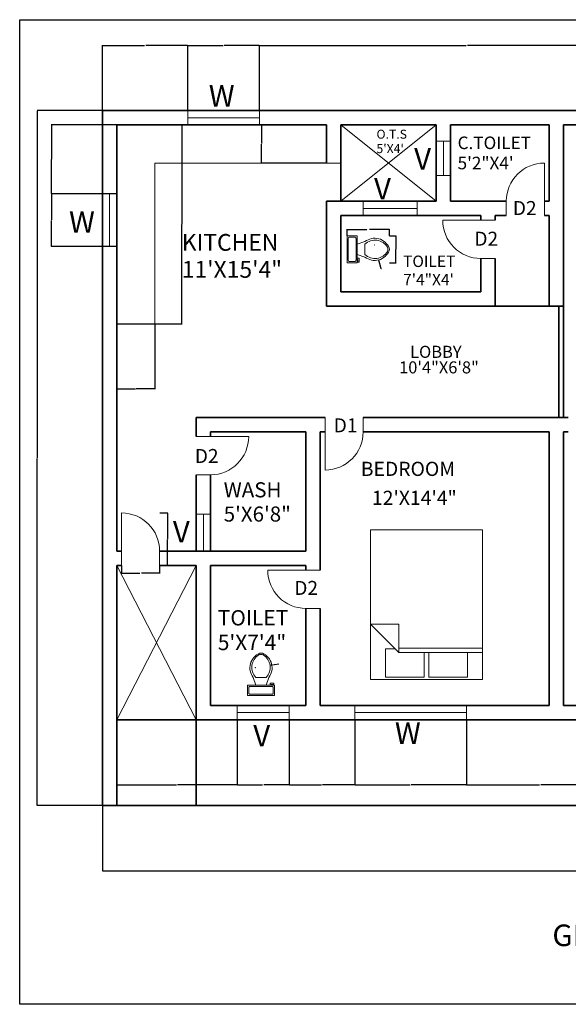
# Model space of a CAD drawing. Units: feet. Extents: x 1755 to 2628, y 1710 to 2329.
# Tile 1 of 4: x 1755 to 2100, y 1710 to 2329. Entities that reach past the tile are written whole.
import ezdxf

# ---------------------------------------------------------------- set-up
doc = ezdxf.new("R2010")
doc.units = ezdxf.units.FT
for name, color, linetype, lineweight in [('A-ANNO-DIMS', 2, 'Continuous', 18), ('A-ANNO-TEXT', 7, 'Continuous', 18), ('A-ANNO-TTLB', 7, 'Continuous', 25), ('A-AREA-IDEN', 7, 'Continuous', 18), ('A-DOOR', 3, 'Continuous', 18), ('A-FLOR-FIXT', 9, 'Continuous', 18), ('A-FLOR-OPEN', 8, 'Continuous', 13), ('A-FURN', 8, 'Continuous', 18), ('A-GLAZ', 4, 'Continuous', 18), ('A-WALL', 7, 'Continuous', 35)]:
    doc.layers.add(name, color=color, linetype=linetype, lineweight=lineweight)
doc.styles.get("Standard").update_dxf_attribs({"font": 'arial.ttf'})
doc.dimstyles.get("Standard").update_dxf_attribs({"dimtxt": 0.18, "dimasz": 0.18, "dimexe": 0.18, "dimexo": 0.0625, "dimgap": 0.09, "dimtad": 0, "dimtih": 1, "dimtoh": 1, "dimdec": 4, "dimzin": 0, "dimdsep": 46, "dimtxsty": 'Standard', "dimcen": 0.09, "dimadec": 0, "dimazin": 0, "dimtfac": 1, "dimtdec": 4, "dimtofl": 0, "dimtmove": 0, "dimatfit": 3, "dimfxl": 1, "dimtolj": 1, "dimtzin": 0, "dimarcsym": 0})

# ---------------------------------------------------------------- blocks, each defined once
blk = doc.blocks.new('Toilet - top')
for p, q in [((9.5, -6), (9.5, -2)), ((-10, -8.5), (-8, -8.5)), ((-10, -9.5), (-10, -8.5)), ((-7, -9.5), (-10, -9.5)), ((-8, -8.5), (-8, -8)), ((-7, -8), (-7, -9.5)), ((-4, -8), (-6, -14)), ((4, -14), (-4, -14)), ((4, -8), (6, -14))]:
    blk.add_line(p, q)
blk.add_lwpolyline([(10.5, -8), (10.5, 0), (-10.5, 0), (-10.5, -8)], close=True)
for points in [[(-9.5, -2), (-9.5, -6)], [(8.5, -1), (-8.5, -1)], [(-8.5, -7), (8.5, -7)]]:
    blk.add_lwpolyline(points)
for centre, radius, start, end in [((-8.62, -1.88), 0.884, 81.8699, 188.1301), ((-8.62, -6.12), 0.884, 171.8699, 278.1301), ((8.62, -1.88), 0.884, 351.8699, 98.1301), ((8.62, -6.12), 0.884, 261.8699, 8.1301), ((3.52, -21.58), 12.17, 141.46911, 247.97143), ((4.2, -21.82), 11.33, 136.36773, 238.94682), ((-3.52, -21.58), 12.17, 292.02843, 38.53071), ((-4.2, -21.82), 11.33, 301.05301, 43.63209), ((0, -27.88), 4, 245.73182, 294.26817), ((0, -29), 4, 254.86053, 285.13947)]:
    blk.add_arc(centre, radius, start, end)
blk = doc.blocks.new('Bed - Queen')
for p, q in [((0, -80.00003), (0, 0)), ((0, 0), (59.99999, 0)), ((59.99999, 0), (59.99999, -80.00003)), ((7.99999, -1.2), (28.79998, -1.2)), ((7.99999, -14.4), (7.99999, -1.2)), ((28.79998, -1.2), (28.79998, -14.4)), ((31.19999, -1.2), (51.99999, -1.2)), ((31.19999, -14.4), (31.19999, -1.2)), ((51.99999, -1.2), (51.99999, -16.4)), ((0, -14.4), (44.8, -14.4)), ((59.99999, -29.6), (44.8, -14.4)), ((44.8, -14.4), (44.8, -29.6)), ((44.8, -16.8), (0, -16.8)), ((51.99999, -16.4), (46.79936, -16.4)), ((44.8, -29.6), (59.99999, -29.6)), ((59.99999, -80.00003), (0, -80.00003))]:
    blk.add_line(p, q)
blk = doc.blocks.new('DOOR-SINGLE-SWING')
for p, q in [((0, 33), (0, 0)), ((24, 9), (24, 0))]:
    blk.add_line(p, q)
blk.add_arc((0, 9), 24, 0, 90)
blk = doc.blocks.new('*D8')
at = {"layer": 'A-ANNO-DIMS', "color": 0, "lineweight": -2, "transparency": 16777216}
for p, q in [((1842.95, 2018.82), (1848.02, 2018.82)), ((1847.84, 2018.64), (1847.84, 2002.5)), ((1847.84, 1986), (1847.84, 2002.13)), ((1842.95, 1985.82), (1848.02, 1985.82))]:
    blk.add_line(p, q, dxfattribs=at)
at = {"layer": 'A-ANNO-DIMS', "color": 0, "transparency": 16777216}
for points in [[(1847.81, 2018.64), (1847.87, 2018.64), (1847.84, 2018.82)], [(1847.81, 1986), (1847.87, 1986), (1847.84, 1985.82)]]:
    blk.add_solid(points, dxfattribs=at)
at = {"layer": 'Defpoints', "color": 0, "transparency": 16777216}
for p in [(1842.89, 2018.82), (1847.84, 2018.82), (1842.89, 1985.82)]:
    blk.add_point(p, dxfattribs=at)
at = {"layer": 'A-ANNO-DIMS', "color": 0, "transparency": 16777216, "insert": (1847.84, 2002.32), "char_height": 0.18, "attachment_point": 5}
blk.add_mtext('\\A1;SWING DOOR 33 TYP.', dxfattribs=at)
blk = doc.blocks.new('*D9')
at = {"layer": 'A-ANNO-DIMS', "color": 0, "lineweight": -2, "transparency": 16777216}
for p, q in [((1818.89, 1985.75), (1818.89, 1980.69)), ((1819.07, 1980.87), (1830.36, 1980.87)), ((1842.71, 1980.87), (1831.42, 1980.87)), ((1842.89, 1985.75), (1842.89, 1980.69))]:
    blk.add_line(p, q, dxfattribs=at)
at = {"layer": 'A-ANNO-DIMS', "color": 0, "transparency": 16777216}
for points in [[(1819.07, 1980.9), (1819.07, 1980.84), (1818.89, 1980.87)], [(1842.71, 1980.9), (1842.71, 1980.84), (1842.89, 1980.87)]]:
    blk.add_solid(points, dxfattribs=at)
at = {"layer": 'Defpoints', "color": 0, "transparency": 16777216}
for p in [(1818.89, 1985.82), (1842.89, 1985.82), (1842.89, 1980.87)]:
    blk.add_point(p, dxfattribs=at)
at = {"layer": 'A-ANNO-DIMS', "color": 0, "transparency": 16777216, "insert": (1830.89, 1980.87), "char_height": 0.18, "attachment_point": 5}
blk.add_mtext('\\A1;24 TYP.', dxfattribs=at)
blk = doc.blocks.new('*D12')
at = {"layer": 'A-ANNO-DIMS', "color": 0, "lineweight": -2, "transparency": 16777216}
for p, q in [((1960.72, 2193.1), (1960.72, 2197.22)), ((1960.9, 2197.04), (1973.28, 2197.04)), ((1987.22, 2197.04), (1974.84, 2197.04)), ((1987.4, 2193.1), (1987.4, 2197.22))]:
    blk.add_line(p, q, dxfattribs=at)
at = {"layer": 'A-ANNO-DIMS', "color": 0, "transparency": 16777216}
for points in [[(1960.9, 2197.07), (1960.9, 2197.01), (1960.72, 2197.04)], [(1987.22, 2197.07), (1987.22, 2197.01), (1987.4, 2197.04)]]:
    blk.add_solid(points, dxfattribs=at)
at = {"layer": 'Defpoints', "color": 0, "transparency": 16777216}
for p in [(1960.72, 2197.04), (1960.72, 2193.04), (1987.4, 2193.04)]:
    blk.add_point(p, dxfattribs=at)
at = {"layer": 'A-ANNO-DIMS', "color": 0, "transparency": 16777216, "insert": (1974.06, 2197.04), "char_height": 0.18, "attachment_point": 5}
blk.add_mtext('\\A1;WC 27 TYP.', dxfattribs=at)
blk = doc.blocks.new('*D13')
at = {"layer": 'A-ANNO-DIMS', "color": 0, "lineweight": -2, "transparency": 16777216}
for p, q in [((1987.47, 2193.04), (1991.58, 2193.04)), ((1991.4, 2192.86), (1991.4, 2184.74)), ((1991.4, 2176.26), (1991.4, 2184.38)), ((1987.47, 2176.08), (1991.58, 2176.08))]:
    blk.add_line(p, q, dxfattribs=at)
at = {"layer": 'A-ANNO-DIMS', "color": 0, "transparency": 16777216}
for points in [[(1991.37, 2192.86), (1991.43, 2192.86), (1991.4, 2193.04)], [(1991.37, 2176.26), (1991.43, 2176.26), (1991.4, 2176.08)]]:
    blk.add_solid(points, dxfattribs=at)
at = {"layer": 'Defpoints', "color": 0, "transparency": 16777216}
for p in [(1987.4, 2193.04), (1991.4, 2193.04), (1987.4, 2176.08)]:
    blk.add_point(p, dxfattribs=at)
at = {"layer": 'A-ANNO-DIMS', "color": 0, "transparency": 16777216, "insert": (1991.4, 2184.56), "char_height": 0.18, "attachment_point": 5}
blk.add_mtext('\\A1;17 TYP.', dxfattribs=at)
blk = doc.blocks.new('*D22')
at = {"layer": 'A-ANNO-DIMS', "color": 0, "lineweight": -2, "transparency": 16777216}
for p, q in [((1806.89, 1834.75), (1806.89, 1793.69)), ((2548.89, 1834.75), (2548.89, 1793.69)), ((1807.07, 1793.87), (2177.6, 1793.87)), ((2548.71, 1793.87), (2178.18, 1793.87))]:
    blk.add_line(p, q, dxfattribs=at)
at = {"layer": 'A-ANNO-DIMS', "color": 0, "transparency": 16777216}
for points in [[(1807.07, 1793.9), (1807.07, 1793.84), (1806.89, 1793.87)], [(2548.71, 1793.9), (2548.71, 1793.84), (2548.89, 1793.87)]]:
    blk.add_solid(points, dxfattribs=at)
at = {"layer": 'Defpoints', "color": 0, "transparency": 16777216}
for p in [(1806.89, 1834.82), (2548.89, 1834.82), (2548.89, 1793.87)]:
    blk.add_point(p, dxfattribs=at)
at = {"layer": 'A-ANNO-DIMS', "color": 0, "transparency": 16777216, "insert": (2177.89, 1793.87), "char_height": 0.18, "attachment_point": 5}
blk.add_mtext('\\A1;742', dxfattribs=at)
blk = doc.blocks.new('*D23')
at = {"layer": 'A-ANNO-DIMS', "color": 0, "lineweight": -2, "transparency": 16777216}
for p, q in [((1806.83, 2271.82), (1765.76, 2271.82)), ((1765.94, 2271.64), (1765.94, 2053.5)), ((1765.94, 1835), (1765.94, 2053.13)), ((1806.83, 1834.82), (1765.76, 1834.82))]:
    blk.add_line(p, q, dxfattribs=at)
at = {"layer": 'A-ANNO-DIMS', "color": 0, "transparency": 16777216}
for points in [[(1765.91, 2271.64), (1765.97, 2271.64), (1765.94, 2271.82)], [(1765.91, 1835), (1765.97, 1835), (1765.94, 1834.82)]]:
    blk.add_solid(points, dxfattribs=at)
at = {"layer": 'Defpoints', "color": 0, "transparency": 16777216}
for p in [(1765.94, 2271.82), (1806.89, 2271.82), (1806.89, 1834.82)]:
    blk.add_point(p, dxfattribs=at)
at = {"layer": 'A-ANNO-DIMS', "color": 0, "transparency": 16777216, "insert": (1765.94, 2053.32), "char_height": 0.18, "attachment_point": 5}
blk.add_mtext('\\A1;437', dxfattribs=at)
blk = doc.blocks.new('*D24')
at = {"layer": 'A-ANNO-DIMS', "color": 0, "lineweight": -2, "transparency": 16777216}
for p, q in [((1806.89, 2271.88), (1806.89, 2312.95)), ((1807.07, 2312.77), (1833.36, 2312.77)), ((1860.43, 2312.77), (1834.14, 2312.77)), ((1860.61, 2271.88), (1860.61, 2312.95))]:
    blk.add_line(p, q, dxfattribs=at)
at = {"layer": 'A-ANNO-DIMS', "color": 0, "transparency": 16777216}
for points in [[(1807.07, 2312.8), (1807.07, 2312.74), (1806.89, 2312.77)], [(1860.43, 2312.8), (1860.43, 2312.74), (1860.61, 2312.77)]]:
    blk.add_solid(points, dxfattribs=at)
at = {"layer": 'Defpoints', "color": 0, "transparency": 16777216}
for p in [(1860.61, 2312.77), (1806.89, 2271.82), (1860.61, 2271.82)]:
    blk.add_point(p, dxfattribs=at)
at = {"layer": 'A-ANNO-DIMS', "color": 0, "transparency": 16777216, "insert": (1833.75, 2312.77), "char_height": 0.18, "attachment_point": 5}
blk.add_mtext('\\A1;53.72', dxfattribs=at)
blk = doc.blocks.new('*D25')
at = {"layer": 'A-ANNO-DIMS', "color": 0, "lineweight": -2, "transparency": 16777216}
for p, q in [((1860.61, 2271.88), (1860.61, 2312.95)), ((1860.79, 2312.77), (1882.75, 2312.77)), ((1905.51, 2312.77), (1883.55, 2312.77)), ((1905.69, 2271.88), (1905.69, 2312.95))]:
    blk.add_line(p, q, dxfattribs=at)
at = {"layer": 'A-ANNO-DIMS', "color": 0, "transparency": 16777216}
for points in [[(1860.79, 2312.8), (1860.79, 2312.74), (1860.61, 2312.77)], [(1905.51, 2312.8), (1905.51, 2312.74), (1905.69, 2312.77)]]:
    blk.add_solid(points, dxfattribs=at)
at = {"layer": 'Defpoints', "color": 0, "transparency": 16777216}
for p in [(1905.69, 2312.77), (1860.61, 2271.82), (1905.69, 2271.82)]:
    blk.add_point(p, dxfattribs=at)
at = {"layer": 'A-ANNO-DIMS', "color": 0, "transparency": 16777216, "insert": (1883.15, 2312.77), "char_height": 0.18, "attachment_point": 5}
blk.add_mtext('\\A1;45.07', dxfattribs=at)
blk = doc.blocks.new('*D26')
at = {"layer": 'A-ANNO-DIMS', "color": 0, "lineweight": -2, "transparency": 16777216}
for p, q in [((1905.69, 2271.88), (1905.69, 2312.95)), ((1905.87, 2312.77), (2035.59, 2312.77)), ((2166.25, 2312.77), (2036.53, 2312.77)), ((2166.43, 2271.88), (2166.43, 2312.95))]:
    blk.add_line(p, q, dxfattribs=at)
at = {"layer": 'A-ANNO-DIMS', "color": 0, "transparency": 16777216}
for points in [[(1905.87, 2312.8), (1905.87, 2312.74), (1905.69, 2312.77)], [(2166.25, 2312.8), (2166.25, 2312.74), (2166.43, 2312.77)]]:
    blk.add_solid(points, dxfattribs=at)
at = {"layer": 'Defpoints', "color": 0, "transparency": 16777216}
for p in [(2166.43, 2312.77), (1905.69, 2271.82), (2166.43, 2271.82)]:
    blk.add_point(p, dxfattribs=at)
at = {"layer": 'A-ANNO-DIMS', "color": 0, "transparency": 16777216, "insert": (2036.06, 2312.77), "char_height": 0.18, "attachment_point": 5}
blk.add_mtext('\\A1;260.75', dxfattribs=at)
blk = doc.blocks.new('*D36')
at = {"layer": 'A-ANNO-DIMS', "color": 0, "lineweight": -2, "transparency": 16777216}
for p, q in [((1815.89, 1888.75), (1815.89, 1847.69)), ((1891.73, 1888.75), (1891.73, 1847.69)), ((1816.07, 1847.87), (1853.42, 1847.87)), ((1891.55, 1847.87), (1854.2, 1847.87))]:
    blk.add_line(p, q, dxfattribs=at)
at = {"layer": 'A-ANNO-DIMS', "color": 0, "transparency": 16777216}
for points in [[(1816.07, 1847.9), (1816.07, 1847.84), (1815.89, 1847.87)], [(1891.55, 1847.9), (1891.55, 1847.84), (1891.73, 1847.87)]]:
    blk.add_solid(points, dxfattribs=at)
at = {"layer": 'Defpoints', "color": 0, "transparency": 16777216}
for p in [(1815.89, 1888.82), (1891.73, 1888.82), (1815.89, 1847.87)]:
    blk.add_point(p, dxfattribs=at)
at = {"layer": 'A-ANNO-DIMS', "color": 0, "transparency": 16777216, "insert": (1853.81, 1847.87), "char_height": 0.18, "attachment_point": 5}
blk.add_mtext('\\A1;75.84', dxfattribs=at)
blk = doc.blocks.new('*D37')
at = {"layer": 'A-ANNO-DIMS', "color": 0, "lineweight": -2, "transparency": 16777216}
for p, q in [((1891.73, 1888.75), (1891.73, 1847.69)), ((1924.29, 1888.75), (1924.29, 1847.69)), ((1891.91, 1847.87), (1907.62, 1847.87)), ((1924.11, 1847.87), (1908.4, 1847.87))]:
    blk.add_line(p, q, dxfattribs=at)
at = {"layer": 'A-ANNO-DIMS', "color": 0, "transparency": 16777216}
for points in [[(1891.91, 1847.9), (1891.91, 1847.84), (1891.73, 1847.87)], [(1924.11, 1847.9), (1924.11, 1847.84), (1924.29, 1847.87)]]:
    blk.add_solid(points, dxfattribs=at)
at = {"layer": 'Defpoints', "color": 0, "transparency": 16777216}
for p in [(1891.73, 1888.82), (1924.29, 1888.82), (1891.73, 1847.87)]:
    blk.add_point(p, dxfattribs=at)
at = {"layer": 'A-ANNO-DIMS', "color": 0, "transparency": 16777216, "insert": (1908.01, 1847.87), "char_height": 0.18, "attachment_point": 5}
blk.add_mtext('\\A1;32.56', dxfattribs=at)
blk = doc.blocks.new('*D38')
at = {"layer": 'A-ANNO-DIMS', "color": 0, "lineweight": -2, "transparency": 16777216}
for p, q in [((1924.29, 1888.75), (1924.29, 1847.69)), ((1965.72, 1888.75), (1965.72, 1847.69)), ((1924.47, 1847.87), (1944.61, 1847.87)), ((1965.54, 1847.87), (1945.4, 1847.87))]:
    blk.add_line(p, q, dxfattribs=at)
at = {"layer": 'A-ANNO-DIMS', "color": 0, "transparency": 16777216}
for points in [[(1924.47, 1847.9), (1924.47, 1847.84), (1924.29, 1847.87)], [(1965.54, 1847.9), (1965.54, 1847.84), (1965.72, 1847.87)]]:
    blk.add_solid(points, dxfattribs=at)
at = {"layer": 'Defpoints', "color": 0, "transparency": 16777216}
for p in [(1924.29, 1888.82), (1965.72, 1888.82), (1924.29, 1847.87)]:
    blk.add_point(p, dxfattribs=at)
at = {"layer": 'A-ANNO-DIMS', "color": 0, "transparency": 16777216, "insert": (1945, 1847.87), "char_height": 0.18, "attachment_point": 5}
blk.add_mtext('\\A1;41.43', dxfattribs=at)
blk = doc.blocks.new('*D39')
at = {"layer": 'A-ANNO-DIMS', "color": 0, "lineweight": -2, "transparency": 16777216}
for p, q in [((1965.72, 1888.75), (1965.72, 1847.69)), ((2035.77, 1888.75), (2035.77, 1847.69)), ((1965.9, 1847.87), (2000.35, 1847.87)), ((2035.59, 1847.87), (2001.14, 1847.87))]:
    blk.add_line(p, q, dxfattribs=at)
at = {"layer": 'A-ANNO-DIMS', "color": 0, "transparency": 16777216}
for points in [[(1965.9, 1847.9), (1965.9, 1847.84), (1965.72, 1847.87)], [(2035.59, 1847.9), (2035.59, 1847.84), (2035.77, 1847.87)]]:
    blk.add_solid(points, dxfattribs=at)
at = {"layer": 'Defpoints', "color": 0, "transparency": 16777216}
for p in [(1965.72, 1888.82), (2035.77, 1888.82), (1965.72, 1847.87)]:
    blk.add_point(p, dxfattribs=at)
at = {"layer": 'A-ANNO-DIMS', "color": 0, "transparency": 16777216, "insert": (2000.75, 1847.87), "char_height": 0.18, "attachment_point": 5}
blk.add_mtext('\\A1;70.06', dxfattribs=at)
blk = doc.blocks.new('*D40')
at = {"layer": 'A-ANNO-DIMS', "color": 0, "lineweight": -2, "transparency": 16777216}
for p, q in [((2035.77, 1888.75), (2035.77, 1847.69)), ((2128.5, 1888.75), (2128.5, 1847.69)), ((2035.95, 1847.87), (2081.75, 1847.87)), ((2128.32, 1847.87), (2082.53, 1847.87))]:
    blk.add_line(p, q, dxfattribs=at)
at = {"layer": 'A-ANNO-DIMS', "color": 0, "transparency": 16777216}
for points in [[(2035.95, 1847.9), (2035.95, 1847.84), (2035.77, 1847.87)], [(2128.32, 1847.9), (2128.32, 1847.84), (2128.5, 1847.87)]]:
    blk.add_solid(points, dxfattribs=at)
at = {"layer": 'Defpoints', "color": 0, "transparency": 16777216}
for p in [(2035.77, 1888.82), (2128.5, 1888.82), (2035.77, 1847.87)]:
    blk.add_point(p, dxfattribs=at)
at = {"layer": 'A-ANNO-DIMS', "color": 0, "transparency": 16777216, "insert": (2082.14, 1847.87), "char_height": 0.18, "attachment_point": 5}
blk.add_mtext('\\A1;92.73', dxfattribs=at)
blk = doc.blocks.new('*D49')
at = {"layer": 'A-ANNO-DIMS', "color": 0, "lineweight": -2, "transparency": 16777216}
for p, q in [((1815.83, 2219.52), (1774.76, 2219.52)), ((1774.94, 2219.34), (1774.94, 2203.14)), ((1774.94, 2186.58), (1774.94, 2202.78)), ((1815.83, 2186.4), (1774.76, 2186.4))]:
    blk.add_line(p, q, dxfattribs=at)
at = {"layer": 'A-ANNO-DIMS', "color": 0, "transparency": 16777216}
for points in [[(1774.91, 2219.34), (1774.97, 2219.34), (1774.94, 2219.52)], [(1774.91, 2186.58), (1774.97, 2186.58), (1774.94, 2186.4)]]:
    blk.add_solid(points, dxfattribs=at)
at = {"layer": 'Defpoints', "color": 0, "transparency": 16777216}
for p in [(1774.94, 2219.52), (1815.89, 2219.52), (1815.89, 2186.4)]:
    blk.add_point(p, dxfattribs=at)
at = {"layer": 'A-ANNO-DIMS', "color": 0, "transparency": 16777216, "insert": (1774.94, 2202.96), "char_height": 0.18, "attachment_point": 5}
blk.add_mtext('\\A1;33.12', dxfattribs=at)
blk = doc.blocks.new('*D50')
at = {"layer": 'A-ANNO-DIMS', "color": 0, "lineweight": -2, "transparency": 16777216}
for p, q in [((1815.83, 2262.82), (1774.76, 2262.82)), ((1774.94, 2262.64), (1774.94, 2241.35)), ((1774.94, 2219.7), (1774.94, 2240.98)), ((1815.83, 2219.52), (1774.76, 2219.52))]:
    blk.add_line(p, q, dxfattribs=at)
at = {"layer": 'A-ANNO-DIMS', "color": 0, "transparency": 16777216}
for points in [[(1774.91, 2262.64), (1774.97, 2262.64), (1774.94, 2262.82)], [(1774.91, 2219.7), (1774.97, 2219.7), (1774.94, 2219.52)]]:
    blk.add_solid(points, dxfattribs=at)
at = {"layer": 'Defpoints', "color": 0, "transparency": 16777216}
for p in [(1774.94, 2262.82), (1815.89, 2262.82), (1815.89, 2219.52)]:
    blk.add_point(p, dxfattribs=at)
at = {"layer": 'A-ANNO-DIMS', "color": 0, "transparency": 16777216, "insert": (1774.94, 2241.17), "char_height": 0.18, "attachment_point": 5}
blk.add_mtext('\\A1;43.3', dxfattribs=at)
blk = doc.blocks.new('*D51')
at = {"layer": 'A-ANNO-DIMS', "color": 0, "lineweight": -2, "transparency": 16777216}
for p, q in [((1815.89, 2137.71), (1815.89, 2096.64)), ((1839.89, 2137.71), (1839.89, 2096.64)), ((1816.07, 2096.82), (1827.67, 2096.82)), ((1839.71, 2096.82), (1828.11, 2096.82))]:
    blk.add_line(p, q, dxfattribs=at)
at = {"layer": 'A-ANNO-DIMS', "color": 0, "transparency": 16777216}
for points in [[(1816.07, 2096.85), (1816.07, 2096.79), (1815.89, 2096.82)], [(1839.71, 2096.85), (1839.71, 2096.79), (1839.89, 2096.82)]]:
    blk.add_solid(points, dxfattribs=at)
at = {"layer": 'Defpoints', "color": 0, "transparency": 16777216}
for p in [(1815.89, 2137.77), (1839.89, 2137.77), (1815.89, 2096.82)]:
    blk.add_point(p, dxfattribs=at)
at = {"layer": 'A-ANNO-DIMS', "color": 0, "transparency": 16777216, "insert": (1827.89, 2096.82), "char_height": 0.18, "attachment_point": 5}
blk.add_mtext('\\A1;24', dxfattribs=at)
blk = doc.blocks.new('*D52')
at = {"layer": 'A-ANNO-DIMS', "color": 0, "lineweight": -2, "transparency": 16777216}
for p, q in [((1815.95, 2262.82), (1857.02, 2262.82)), ((1856.84, 2262.64), (1856.84, 2200.48)), ((1856.84, 2137.95), (1856.84, 2200.11)), ((1815.95, 2137.77), (1857.02, 2137.77))]:
    blk.add_line(p, q, dxfattribs=at)
at = {"layer": 'A-ANNO-DIMS', "color": 0, "transparency": 16777216}
for points in [[(1856.81, 2262.64), (1856.87, 2262.64), (1856.84, 2262.82)], [(1856.81, 2137.95), (1856.87, 2137.95), (1856.84, 2137.77)]]:
    blk.add_solid(points, dxfattribs=at)
at = {"layer": 'Defpoints', "color": 0, "transparency": 16777216}
for p in [(1815.89, 2262.82), (1815.89, 2137.77), (1856.84, 2137.77)]:
    blk.add_point(p, dxfattribs=at)
at = {"layer": 'A-ANNO-DIMS', "color": 0, "transparency": 16777216, "insert": (1856.84, 2200.3), "char_height": 0.18, "attachment_point": 5}
blk.add_mtext('\\A1;125.04', dxfattribs=at)
blk = doc.blocks.new('*D53')
at = {"layer": 'A-ANNO-DIMS', "color": 0, "lineweight": -2, "transparency": 16777216}
for p, q in [((1947.83, 2262.82), (1906.76, 2262.82)), ((1906.94, 2262.64), (1906.94, 2251)), ((1906.94, 2239), (1906.94, 2250.64)), ((1947.83, 2238.82), (1906.76, 2238.82))]:
    blk.add_line(p, q, dxfattribs=at)
at = {"layer": 'A-ANNO-DIMS', "color": 0, "transparency": 16777216}
for points in [[(1906.91, 2262.64), (1906.97, 2262.64), (1906.94, 2262.82)], [(1906.91, 2239), (1906.97, 2239), (1906.94, 2238.82)]]:
    blk.add_solid(points, dxfattribs=at)
at = {"layer": 'Defpoints', "color": 0, "transparency": 16777216}
for p in [(1906.94, 2262.82), (1947.89, 2262.82), (1947.89, 2238.82)]:
    blk.add_point(p, dxfattribs=at)
at = {"layer": 'A-ANNO-DIMS', "color": 0, "transparency": 16777216, "insert": (1906.94, 2250.82), "char_height": 0.18, "attachment_point": 5}
blk.add_mtext('\\A1;24', dxfattribs=at)
blk = doc.blocks.new('*D59')
at = {"layer": 'A-ANNO-DIMS', "color": 0, "lineweight": -2, "transparency": 16777216}
for p, q in [((1978.05, 2187.4), (1978.23, 2187.4)), ((1978.14, 2187.31), (1978.14, 2187.49)), ((1982.14, 2172.2), (1980.69, 2177.73)), ((1982.32, 2172.2), (1982.14, 2172.2))]:
    blk.add_line(p, q, dxfattribs=at)
at = {"layer": 'A-ANNO-DIMS', "color": 0, "transparency": 16777216}
blk.add_solid([(1980.72, 2177.73), (1980.66, 2177.72), (1980.64, 2177.9)], dxfattribs=at)
at = {"layer": 'Defpoints', "color": 0, "transparency": 16777216}
for p in [(1978.14, 2187.4), (1980.64, 2177.9)]:
    blk.add_point(p, dxfattribs=at)
at = {"layer": 'A-ANNO-DIMS', "color": 0, "transparency": 16777216, "insert": (1983, 2172.2), "char_height": 0.18, "attachment_point": 5}
blk.add_mtext('\\A1;4X R9.826', dxfattribs=at)
blk = doc.blocks.new('*D60')
at = {"layer": 'A-ANNO-DIMS', "color": 0, "lineweight": -2, "transparency": 16777216}
for p, q in [((1903.16, 1921.71), (1903.34, 1921.71)), ((1903.25, 1921.62), (1903.25, 1921.8)), ((1917.75, 1923.66), (1912.49, 1922.96))]:
    blk.add_line(p, q, dxfattribs=at)
at = {"layer": 'A-ANNO-DIMS', "color": 0, "transparency": 16777216}
blk.add_solid([(1912.49, 1922.99), (1912.5, 1922.93), (1912.31, 1922.93)], dxfattribs=at)
at = {"layer": 'Defpoints', "color": 0, "transparency": 16777216}
for p in [(1903.25, 1921.71), (1912.31, 1922.93)]:
    blk.add_point(p, dxfattribs=at)
at = {"layer": 'A-ANNO-DIMS', "color": 0, "transparency": 16777216, "insert": (1918.43, 1923.66), "char_height": 0.18, "attachment_point": 5}
blk.add_mtext('\\A1;4X R9.148', dxfattribs=at)

msp = doc.modelspace()

# ---------------------------------------------------------------- linework, layer by layer
at = {"layer": 'A-ANNO-TTLB'}
msp.add_lwpolyline([(1754.8706, 2328.9307), (2627.7013, 2328.9307), (2627.7013, 1709.9251), (1754.8706, 1709.9251)], close=True, dxfattribs=at)
at = {"layer": 'A-FLOR-FIXT'}
for p, q in [((1839.8905, 2238.8157), (1956.8905, 2238.8157)), ((1839.8905, 2137.7746), (1839.8905, 2238.8157)), ((1815.8905, 2137.7746), (1839.8905, 2137.7746))]:
    msp.add_line(p, q, dxfattribs=at)
at = {"layer": 'A-FLOR-OPEN'}
for p, q in [((1956.8905, 2262.8157), (2016.8905, 2214.8157)), ((1956.8905, 2214.8157), (2016.8905, 2262.8157)), ((1815.8905, 1985.8157), (1865.8905, 1888.8157)), ((1865.8905, 1985.8157), (1815.8905, 1888.8157))]:
    msp.add_line(p, q, dxfattribs=at)
at = {"layer": 'A-GLAZ'}
for p, q in [((1860.6124, 2271.8157), (1860.6124, 2262.8157)), ((1905.6851, 2271.8157), (1905.6851, 2262.8157)), ((1860.6124, 2267.3157), (1905.6851, 2267.3157)), ((2016.8905, 2252.4841), (2025.8905, 2252.4841)), ((2021.3905, 2252.4841), (2021.3905, 2230.9614)), ((2016.8905, 2230.9614), (2025.8905, 2230.9614)), ((1806.8905, 2219.5181), (1815.8905, 2219.5181)), ((1811.3905, 2219.5181), (1811.3905, 2186.3991)), ((1970.8608, 2214.8157), (1970.8608, 2205.8157)), ((1970.8608, 2210.3157), (2004.908, 2210.3157)), ((2004.908, 2214.8157), (2004.908, 2205.8157)), ((1806.8905, 2186.3991), (1815.8905, 2186.3991)), ((1865.8905, 2018.1107), (1874.8905, 2018.1107)), ((1870.3905, 2018.1107), (1870.3905, 1994.8157)), ((1891.7318, 1897.8157), (1891.7318, 1888.8157)), ((1924.2905, 1897.8157), (1924.2905, 1888.8157)), ((1965.7178, 1897.8157), (1965.7178, 1888.8157)), ((2035.7745, 1897.8157), (2035.7745, 1888.8157)), ((1891.7318, 1893.3157), (1924.2905, 1893.3157)), ((1965.7178, 1893.3157), (2035.7745, 1893.3157))]:
    msp.add_line(p, q, dxfattribs=at)
at = {"layer": 'A-WALL'}
for p, q in [((1806.8905, 2271.8157), (1947.8905, 2271.8157)), ((1806.8905, 2078.8157), (1806.8905, 2271.8157)), ((1806.8905, 2271.8157), (2096.8905, 2271.8157)), ((2025.8905, 2271.8157), (2096.8905, 2271.8157)), ((2096.8905, 2271.8157), (2548.8905, 2271.8157)), ((1815.8905, 2262.8157), (1947.8905, 2262.8157)), ((1815.8905, 2069.8157), (1815.8905, 2262.8157)), ((1947.8905, 2262.8157), (1947.8905, 2238.8157)), ((1956.8905, 2262.8157), (1956.8905, 2214.8157)), ((1956.8905, 2262.8157), (2016.8905, 2262.8157)), ((2016.8905, 2262.8157), (2016.8905, 2214.8157)), ((2025.8905, 2262.8157), (2025.8905, 2214.8157)), ((2025.8905, 2262.8157), (2087.8905, 2262.8157)), ((2087.8905, 2262.8157), (2087.8905, 2214.8157)), ((2096.8905, 2262.8157), (2096.8905, 2214.8157)), ((2096.8905, 2262.8157), (2378.8905, 2262.8157)), ((2016.8905, 2214.8157), (1947.8905, 2214.8157)), ((1947.8905, 2214.8157), (1947.8905, 2148.8157)), ((1956.8905, 2214.8157), (2016.8905, 2214.8157)), ((2060.8905, 2214.8157), (2025.8905, 2214.8157)), ((2087.8905, 2214.8157), (2084.8905, 2214.8157)), ((2096.8905, 2214.8157), (2096.8905, 2078.8157)), ((1956.8905, 2205.8157), (1956.8905, 2157.8157)), ((1956.8905, 2205.8157), (2044.8905, 2205.8157)), ((2044.8905, 2205.8157), (2044.8905, 2202.8157)), ((2053.8905, 2205.8157), (2053.8905, 2202.8157)), ((2053.8905, 2205.8157), (2060.8905, 2205.8157)), ((2084.8905, 2205.8157), (2087.8905, 2205.8157)), ((2087.8905, 2205.8157), (2087.8905, 2148.8157)), ((2044.8905, 2178.8157), (2044.8905, 2157.8157)), ((2053.8905, 2178.8157), (2053.8905, 2148.8157)), ((2044.8905, 2157.8157), (1956.8905, 2157.8157)), ((2096.8905, 2148.8157), (1947.8905, 2148.8157)), ((2093.8905, 2148.8157), (2093.8905, 2078.8157)), ((1806.8905, 2078.8157), (1806.8905, 1888.8157)), ((1946.8905, 2078.8157), (1865.8905, 2078.8157)), ((1865.8905, 2066.8157), (1865.8905, 2078.8157)), ((1946.8905, 2078.8157), (1865.8905, 2078.8157)), ((2096.8905, 2078.8157), (1970.8905, 2078.8157)), ((2099.8905, 2078.8157), (2096.8905, 2078.8157)), ((1815.8905, 2069.8157), (1815.8905, 1994.8157)), ((1874.8905, 2066.8157), (1874.8905, 2069.8157)), ((1934.8905, 2069.8157), (1874.8905, 2069.8157)), ((1934.8905, 2069.8157), (1934.8905, 1994.8157)), ((1943.8905, 2069.8157), (1943.8905, 1982.8157)), ((1946.8905, 2069.8157), (1943.8905, 2069.8157)), ((1946.8905, 2069.8157), (1944.8905, 2069.8157)), ((2087.8905, 2069.8157), (1970.8905, 2069.8157)), ((2087.8905, 1897.8157), (2087.8905, 2069.8157)), ((2096.8905, 1897.8157), (2096.8905, 2069.8157)), ((2099.8905, 2069.8157), (2096.8905, 2069.8157)), ((1865.8905, 1994.8157), (1865.8905, 2042.8157)), ((1874.8905, 1994.8157), (1874.8905, 2042.8157)), ((1815.8905, 1994.8157), (1818.8905, 1994.8157)), ((1842.8905, 1994.8157), (1874.8905, 1994.8157)), ((1874.8905, 1994.8157), (1934.8905, 1994.8157)), ((1815.8905, 1985.8157), (1818.8905, 1985.8157)), ((1815.8905, 1985.8157), (1815.8905, 1888.8157)), ((1815.8905, 1985.8157), (1815.8905, 1834.8157)), ((1842.8905, 1985.8157), (1865.8905, 1985.8157)), ((1865.8905, 1834.8157), (1865.8905, 1985.8157)), ((1874.8905, 1897.8157), (1874.8905, 1985.8157)), ((1874.8905, 1985.8157), (1934.8905, 1985.8157)), ((1934.8905, 1985.8157), (1934.8905, 1982.8157)), ((1934.8905, 1958.8157), (1934.8905, 1897.8157)), ((1943.8905, 1958.8157), (1943.8905, 1897.8157)), ((1934.8905, 1897.8157), (1874.8905, 1897.8157)), ((1943.8905, 1897.8157), (2087.8905, 1897.8157)), ((2096.8905, 1897.8157), (2244.8905, 1897.8157)), ((1806.8905, 1888.8157), (1806.8905, 1834.8157)), ((2096.8905, 1888.8157), (1815.8905, 1888.8157)), ((1943.8905, 1888.8157), (2096.8905, 1888.8157)), ((2096.8905, 1888.8157), (2244.8905, 1888.8157)), ((1806.8905, 1834.8157), (2548.8905, 1834.8157))]:
    msp.add_line(p, q, dxfattribs=at)

# ---------------------------------------------------------------- block references
at = {"layer": 'A-DOOR', "extrusion": (0, 0, -1), "zscale": -1}
msp.add_blockref('DOOR-SINGLE-SWING', (-2084.8901, 2205.816), dxfattribs=at)
for p, rotation in [((-2053.8902, 2202.8152), 270.0000000000007), ((-1946.891, 2078.8153), 180), ((-1943.8902, 1982.8152), 270.0000000000045)]:
    msp.add_blockref('DOOR-SINGLE-SWING', p, dxfattribs=dict(at, rotation=rotation))
at = {"layer": 'A-DOOR', "rotation": 270.0000000000037}
msp.add_blockref('DOOR-SINGLE-SWING', (1865.8909, 2066.8152), dxfattribs=at)
at = {"layer": 'A-DOOR'}
msp.add_blockref('DOOR-SINGLE-SWING', (1818.891, 1985.816), dxfattribs=at)
at = {"layer": 'A-FLOR-FIXT', "xscale": 0.8074435145165587, "yscale": 0.8074435145165587, "zscale": 0.8074435145165587}
for p, rotation in [((1960.7196, 2184.561), 90), ((1906.64, 1904.097), 180)]:
    msp.add_blockref('Toilet - top', p, dxfattribs=dict(at, rotation=rotation))
at = {"layer": 'A-FURN', "xscale": 1.174519185879722, "yscale": 1.174519185879722, "zscale": 1.174519185879722, "rotation": 180}
msp.add_blockref('Bed - Queen', (2045.9481, 1914.1832), dxfattribs=at)

# ---------------------------------------------------------------- texts
at = {"layer": 'A-ANNO-TEXT'}
for s, height, p in [('W', 13.589, (1873.7685, 2274.2821)), ('V', 13.589, (2002.9116, 2234.6686)), ('V', 13.589, (1977.6939, 2215.9093)), ('D2', 8.79691, (2065.0213, 2206.1171)), ('W', 13.589, (1785.8814, 2194.9533)), ('D2', 8.79691, (2040.8371, 2186.837)), ('D1', 8.79691, (1952.3739, 2069.5056)), ('D2', 8.79691, (1865.019, 2050.2479)), ('V', 13.589, (1851.1874, 2000.2852)), ('D2', 8.79691, (1927.5763, 1967.2883)), ('V', 13.589, (1901.7375, 1872.0079)), ('W', 13.589, (1990.8302, 1873.6013))]:
    msp.add_text(s, height=height, dxfattribs=at).set_placement(p)
at = {"layer": 'A-ANNO-TTLB'}
msp.add_text('GROUND FLOOR', height=13.589045, dxfattribs=at).set_placement((2089.8587, 1746.5043))
at = {"layer": 'A-AREA-IDEN'}
for s, height, p in [('O.T.S', 5.6407, (1979.2429, 2254.1156)), ('C.TOILET', 7.90528, (2030.2575, 2247.5755)), ("5'X4'", 5.6407, (1979.2429, 2245.0543)), ('5\'2"X4\'', 7.90528, (2030.2575, 2234.8764)), ('KITCHEN', 10.56023, (1856.8028, 2183.6432)), ('TOILET', 7.16525, (1995.9801, 2173.4596)), ('11\'X15\'4"', 10.56023, (1856.8028, 2166.6791)), ('7\'4"X4\'', 7.16525, (1995.9801, 2161.9493)), ('LOBBY', 7.57521, (2000.412, 2116.3415)), ('10\'4"X6\'8"', 7.57521, (1993.4965, 2106.5553)), ('BEDROOM', 8.93153, (1969.3738, 2042.0849)), ('WASH', 9.48162, (1883.1669, 2028.6328)), ('12\'X14\'4"', 8.93153, (1976.392, 2023.8611)), ('5\'X6\'8"', 9.48162, (1883.1669, 2013.4014)), ('TOILET', 9.64966, (1879.4611, 1948.095)), ('5\'X7\'4"', 9.64966, (1879.4611, 1932.5937))]:
    msp.add_text(s, height=height, dxfattribs=at).set_placement(p)

# ---------------------------------------------------------------- dimensions: what is measured, and where the dimension line sits
at = {"layer": 'A-ANNO-DIMS'}
for base, p1, p2, override, picture, middle in [((1860.6124, 2312.7657), (1806.8905, 2271.8157), (1860.6124, 2271.8157), {"dimdec": 2, "dimlfac": 1, "dimrnd": 0, "dimzin": 0, "dimdsep": 46, "dimlunit": 2}, '*D24', (1833.7515, 2312.7657)), ((1905.6851, 2312.7657), (1860.6124, 2271.8157), (1905.6851, 2271.8157), {"dimdec": 2, "dimlfac": 1, "dimrnd": 0, "dimzin": 0, "dimdsep": 46, "dimlunit": 2}, '*D25', (1883.1488, 2312.7657)), ((2166.4346, 2312.7657), (1905.6851, 2271.8157), (2166.4346, 2271.8157), {"dimdec": 2, "dimlfac": 1, "dimrnd": 0, "dimzin": 0, "dimdsep": 46, "dimlunit": 2}, '*D26', (2036.0599, 2312.7657)), ((2548.8905, 1793.8657), (1806.8905, 1834.8157), (2548.8905, 1834.8157), {"dimdec": 0, "dimlfac": 1, "dimrnd": 0, "dimzin": 0, "dimdsep": 46, "dimlunit": 2}, '*D22', (2177.8905, 1793.8657))]:
    dim = msp.add_linear_dim(base=base, p1=p1, p2=p2, dimstyle='Standard', override=override, dxfattribs=at)
    dim.commit()
    dim.dimension.update_dxf_attribs({"geometry": picture, "text_midpoint": middle})
for base, p1, p2, angle, override, picture, middle in [((1765.9405, 2271.8157), (1806.8905, 1834.8157), (1806.8905, 2271.8157), 90, {"dimdec": 0, "dimlfac": 1, "dimrnd": 0, "dimzin": 0, "dimdsep": 46, "dimlunit": 2}, '*D23', (1765.9405, 2053.3157)), ((1774.9405, 2262.8157), (1815.8905, 2219.5181), (1815.8905, 2262.8157), 90, {"dimdec": 1, "dimlfac": 1, "dimrnd": 0, "dimzin": 0, "dimdsep": 46, "dimlunit": 2}, '*D50', (1774.9405, 2241.1669)), ((1856.8405, 2137.7746), (1815.8905, 2262.8157), (1815.8905, 2137.7746), 270, {"dimdec": 2, "dimlfac": 1, "dimrnd": 0, "dimzin": 0, "dimdsep": 46, "dimlunit": 2}, '*D52', (1856.8405, 2200.2951)), ((1906.9405, 2262.8157), (1947.8905, 2238.8157), (1947.8905, 2262.8157), 90, {"dimdec": 0, "dimlfac": 1, "dimrnd": 0, "dimzin": 0, "dimdsep": 46, "dimlunit": 2}, '*D53', (1906.9405, 2250.8157)), ((1774.9405, 2219.5181), (1815.8905, 2186.3991), (1815.8905, 2219.5181), 90, {"dimdec": 2, "dimlfac": 1, "dimrnd": 0, "dimzin": 0, "dimdsep": 46, "dimlunit": 2}, '*D49', (1774.9405, 2202.9586)), ((1815.8905, 2096.8246), (1839.8905, 2137.7746), (1815.8905, 2137.7746), 180, {"dimdec": 0, "dimlfac": 1, "dimrnd": 0, "dimzin": 0, "dimdsep": 46, "dimlunit": 2}, '*D51', (1827.8905, 2096.8246)), ((1815.8905, 1847.8657), (1891.7318, 1888.8157), (1815.8905, 1888.8157), 180, {"dimdec": 2, "dimlfac": 1, "dimrnd": 0, "dimzin": 0, "dimdsep": 46, "dimlunit": 2}, '*D36', (1853.8111, 1847.8657)), ((1891.7318, 1847.8657), (1924.2905, 1888.8157), (1891.7318, 1888.8157), 180, {"dimdec": 2, "dimlfac": 1, "dimrnd": 0, "dimzin": 0, "dimdsep": 46, "dimlunit": 2}, '*D37', (1908.0111, 1847.8657)), ((1924.2905, 1847.8657), (1965.7178, 1888.8157), (1924.2905, 1888.8157), 180, {"dimdec": 2, "dimlfac": 1, "dimrnd": 0, "dimzin": 0, "dimdsep": 46, "dimlunit": 2}, '*D38', (1945.0041, 1847.8657)), ((1965.7178, 1847.8657), (2035.7745, 1888.8157), (1965.7178, 1888.8157), 180, {"dimdec": 2, "dimlfac": 1, "dimrnd": 0, "dimzin": 0, "dimdsep": 46, "dimlunit": 2}, '*D39', (2000.7461, 1847.8657)), ((2035.7745, 1847.8657), (2128.5041, 1888.8157), (2035.7745, 1888.8157), 180, {"dimdec": 2, "dimlfac": 1, "dimrnd": 0, "dimzin": 0, "dimdsep": 46, "dimlunit": 2}, '*D40', (2082.1393, 1847.8657))]:
    dim = msp.add_linear_dim(base=base, p1=p1, p2=p2, angle=angle, dimstyle='Standard', override=override, dxfattribs=at)
    dim.commit()
    dim.dimension.update_dxf_attribs({"geometry": picture, "text_midpoint": middle})
for base, p1, p2, angle, text, picture, middle in [((1960.7196, 2197.0416), (1987.4025, 2193.0391), (1960.7196, 2193.0391), 180, 'WC <> TYP.', '*D12', (1974.061, 2197.0416)), ((1991.405, 2193.0391), (1987.4025, 2176.0828), (1987.4025, 2193.0391), 90, '<> TYP.', '*D13', (1991.405, 2184.561)), ((1847.8405, 2018.8157), (1842.8905, 1985.8157), (1842.8905, 2018.8157), 90, 'SWING DOOR <> TYP.', '*D8', (1847.8405, 2002.3157))]:
    dim = msp.add_linear_dim(base=base, p1=p1, p2=p2, angle=angle, text=text, dimstyle='Standard', override={"dimdec": 0, "dimlfac": 1, "dimrnd": 0, "dimzin": 0, "dimdsep": 46, "dimlunit": 2}, dxfattribs=at)
    dim.commit()
    dim.dimension.update_dxf_attribs({"geometry": picture, "text_midpoint": middle})
for center, mpoint, picture, middle in [((1978.1446, 2187.4028), (1980.6411, 2177.8995), '*D59', (1982.9958, 2172.1975)), ((1903.2488, 1921.7133), (1912.3149, 1922.932), '*D60', (1917.7546, 1923.6632))]:
    dim = msp.add_radius_dim(center=center, mpoint=mpoint, text='4X <>', dimstyle='Standard', override={"dimdec": 3, "dimlfac": 1, "dimrnd": 0, "dimzin": 0, "dimdsep": 46, "dimlunit": 2}, dxfattribs=at)
    dim.commit()
    dim.dimension.update_dxf_attribs({"geometry": picture, "text_midpoint": middle, "dimtype": 164})
dim = msp.add_linear_dim(base=(1842.8905, 1980.8657), p1=(1818.8905, 1985.8157), p2=(1842.8905, 1985.8157), text='<> TYP.', dimstyle='Standard', override={"dimdec": 0, "dimlfac": 1, "dimrnd": 0, "dimzin": 0, "dimdsep": 46, "dimlunit": 2}, dxfattribs=at)
dim.commit()
dim.dimension.update_dxf_attribs({"geometry": '*D9', "text_midpoint": (1830.8905, 1980.8657)})

doc.saveas('drawing.dxf')
